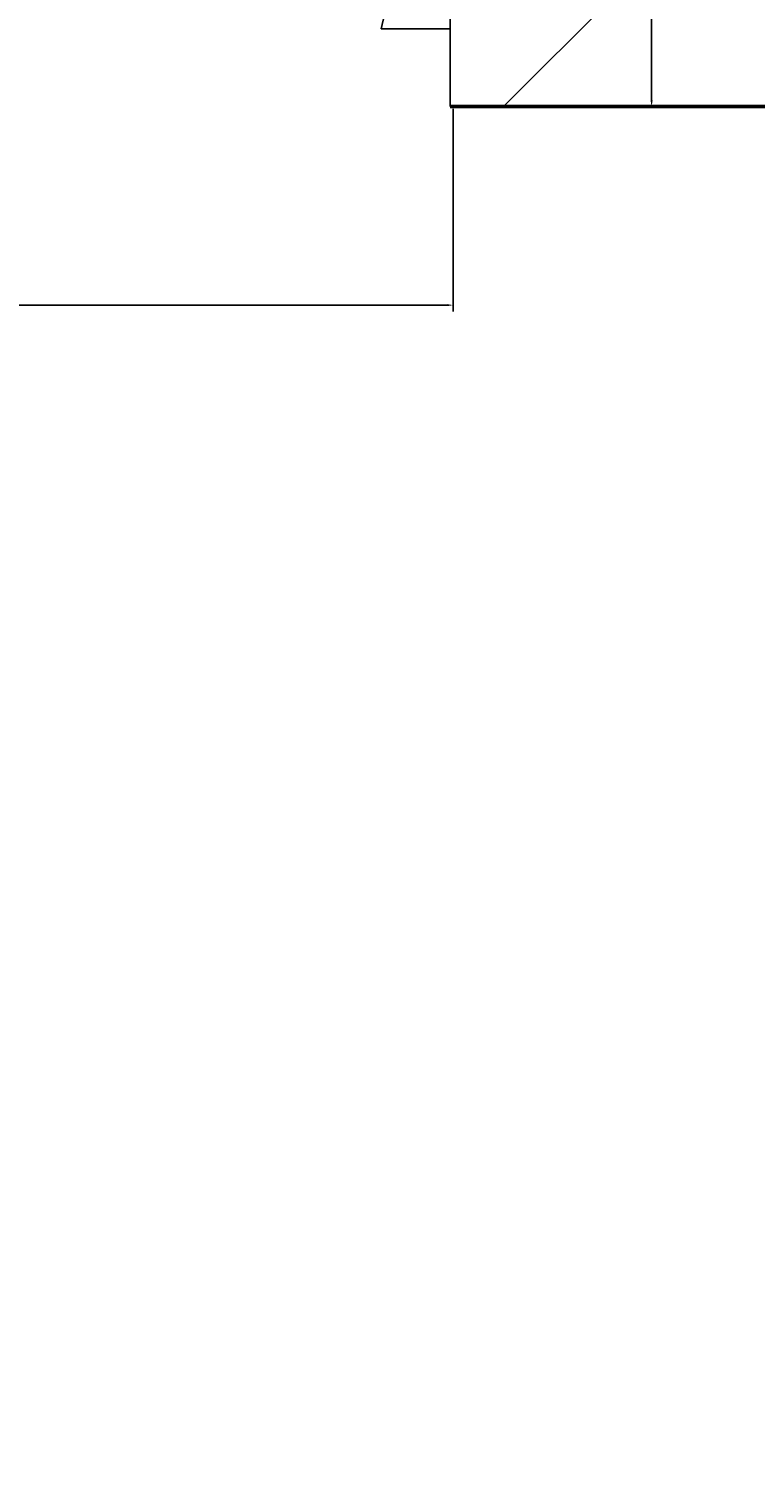
# Model space of a CAD drawing. Units: inches. Extents: x 963 to 2075, y 289 to 2657.
# Tile 93 of 98: x 1788 to 1809, y 2283 to 2325. Entities that reach past the tile are written whole.
import ezdxf

# ---------------------------------------------------------------- set-up
doc = ezdxf.new("R2010")
doc.units = ezdxf.units.IN
for name, color, linetype, lineweight in [('A-ANNO-DIMS', 2, 'Continuous', 18), ('A-DOOR', 4, 'Continuous', 25), ('A-WALL', 7, 'Continuous', 50), ('A-WALL-PATT', 8, 'Continuous', 13)]:
    doc.layers.add(name, color=color, linetype=linetype, lineweight=lineweight)
doc.styles.get("Standard").update_dxf_attribs({"font": 'arial.ttf'})
doc.dimstyles.get("Standard").update_dxf_attribs({"dimtxt": 0.18, "dimasz": 0.18, "dimexe": 0.18, "dimexo": 0.0625, "dimgap": 0.09, "dimtad": 0, "dimtih": 1, "dimtoh": 1, "dimdec": 4, "dimzin": 0, "dimdsep": 46, "dimtxsty": 'Standard', "dimcen": 0.09, "dimadec": 0, "dimazin": 0, "dimtfac": 1, "dimtdec": 4, "dimtofl": 0, "dimtmove": 0, "dimatfit": 3, "dimfxl": 1, "dimtolj": 1, "dimtzin": 0, "dimarcsym": 0})

# ---------------------------------------------------------------- blocks, each defined once
blk = doc.blocks.new('DOOR-3')
for p, q in [((2, 2.25), (2, 38.25)), ((0, 4.5), (0, 0)), ((32.386, 4.5), (32.386, 0)), ((0, 0), (0, 2.25)), ((0, 2.25), (2, 2.25)), ((32.386, 2.25), (30.386, 2.25)), ((32.386, 0), (32.386, 2.25))]:
    blk.add_line(p, q)
blk.add_arc((2, 9.059), 29.191, 346.5105, 90)
blk = doc.blocks.new('*D34')
at = {"layer": 'A-ANNO-DIMS', "color": 0, "lineweight": -2, "transparency": 16777216}
for p, q in [((1800.571, 2361.068), (1806.426, 2361.068)), ((1806.246, 2360.888), (1806.246, 2342.126)), ((1806.246, 2322.998), (1806.246, 2341.759)), ((1800.571, 2322.818), (1806.426, 2322.818))]:
    blk.add_line(p, q, dxfattribs=at)
at = {"layer": 'A-ANNO-DIMS', "color": 0, "transparency": 16777216}
for points in [[(1806.216, 2360.888), (1806.276, 2360.888), (1806.246, 2361.068)], [(1806.216, 2322.998), (1806.276, 2322.998), (1806.246, 2322.818)]]:
    blk.add_solid(points, dxfattribs=at)
at = {"layer": 'Defpoints', "color": 0, "transparency": 16777216}
for p in [(1800.508, 2361.068), (1806.246, 2361.068), (1800.508, 2322.818)]:
    blk.add_point(p, dxfattribs=at)
at = {"layer": 'A-ANNO-DIMS', "color": 0, "transparency": 16777216, "insert": (1806.246, 2341.943), "char_height": 0.18, "attachment_point": 5}
blk.add_mtext('\\A1;DOOR D3 38 TYP.', dxfattribs=at)
blk = doc.blocks.new('*D35')
at = {"layer": 'A-ANNO-DIMS', "color": 0, "lineweight": -2, "transparency": 16777216}
for p, q in [((1768.037, 2322.755), (1768.037, 2316.9)), ((1800.508, 2322.755), (1800.508, 2316.9)), ((1768.217, 2317.08), (1783.745, 2317.08)), ((1800.328, 2317.08), (1784.801, 2317.08))]:
    blk.add_line(p, q, dxfattribs=at)
at = {"layer": 'A-ANNO-DIMS', "color": 0, "transparency": 16777216}
for points in [[(1768.217, 2317.11), (1768.217, 2317.05), (1768.037, 2317.08)], [(1800.328, 2317.11), (1800.328, 2317.05), (1800.508, 2317.08)]]:
    blk.add_solid(points, dxfattribs=at)
at = {"layer": 'Defpoints', "color": 0, "transparency": 16777216}
for p in [(1768.037, 2322.818), (1800.508, 2322.818), (1800.508, 2317.08)]:
    blk.add_point(p, dxfattribs=at)
at = {"layer": 'A-ANNO-DIMS', "color": 0, "transparency": 16777216, "insert": (1784.273, 2317.08), "char_height": 0.18, "attachment_point": 5}
blk.add_mtext('\\A1;32 TYP.', dxfattribs=at)

msp = doc.modelspace()

# ---------------------------------------------------------------- hatches: boundary and pattern name
at = {"layer": 'A-WALL-PATT'}
h = msp.add_hatch(dxfattribs=at)
h.set_pattern_fill('ANSI32', color=256)
h.paths.add_polyline_path([(1296.922, 2558.318), (1203.922, 2558.318), (1203.922, 2493.818), (1191.533, 2493.818), (1191.533, 2489.318), (1211.063, 2489.318), (1211.063, 2492.02), (1211.063, 2493.818), (1208.422, 2493.818), (1208.422, 2553.818), (1292.422, 2553.818), (1292.422, 2538.863), (1296.922, 2538.863)])
h.paths.add_polyline_path([(1442.422, 2558.318), (1349.422, 2558.318), (1349.422, 2538.943), (1353.922, 2538.943), (1353.922, 2553.818), (1437.922, 2553.818), (1437.922, 2493.818), (1434.542, 2493.818), (1434.542, 2489.318), (1448.311, 2489.318), (1448.311, 2491.568), (1448.311, 2493.818), (1442.422, 2493.818)])
h.paths.add_polyline_path([(1415.554, 2491.568), (1415.554, 2493.818), (1340.941, 2493.818), (1340.941, 2489.318), (1371.922, 2489.318), (1371.922, 2378.318), (1367.596, 2378.318), (1367.596, 2373.818), (1371.922, 2373.818), (1371.922, 2355.185), (1376.422, 2355.185), (1376.422, 2489.318), (1415.554, 2489.318)])
h.paths.add_polyline_path([(1304.941, 2491.568), (1304.941, 2493.818), (1296.922, 2493.818), (1296.922, 2514.863), (1292.422, 2514.863), (1292.422, 2493.818), (1232.808, 2493.818), (1232.808, 2489.318), (1256.422, 2489.318), (1256.422, 2327.318), (1253.714, 2327.318), (1253.714, 2322.818), (1328.422, 2322.818), (1328.422, 2331.147), (1323.922, 2331.147), (1323.922, 2327.318), (1260.922, 2327.318), (1260.922, 2373.818), (1323.922, 2373.818), (1323.922, 2357.812), (1328.422, 2357.812), (1328.422, 2373.818), (1346.007, 2373.818), (1346.007, 2376.068), (1346.007, 2378.318), (1260.922, 2378.318), (1260.922, 2489.318), (1304.941, 2489.318)])
h.paths.add_polyline_path([(1226.654, 2327.318), (1124.422, 2327.318), (1124.422, 2347.447), (1119.922, 2347.447), (1119.922, 2322.818), (1163.422, 2322.818), (1163.422, 2305.435), (1165.672, 2305.435), (1167.922, 2305.435), (1167.922, 2322.818), (1226.654, 2322.818), (1226.654, 2325.068)])
h.paths.add_polyline_path([(1095.922, 2489.318), (1124.422, 2489.318), (1131.533, 2489.318), (1131.533, 2491.568), (1131.533, 2493.818), (1119.922, 2493.818), (1091.422, 2493.818), (1091.422, 2417.318), (1095.922, 2417.318), (1119.922, 2417.318), (1119.922, 2407.447), (1124.422, 2407.447), (1124.422, 2421.818), (1095.922, 2421.818)])
h.paths.add_polyline_path([(1512.922, 2558.318), (1508.422, 2558.318), (1508.422, 2493.818), (1503.401, 2493.818), (1503.401, 2489.318), (1508.422, 2489.318), (1508.422, 2327.318), (1376.422, 2327.318), (1376.422, 2330.273), (1371.922, 2330.273), (1371.922, 2298.744), (1376.422, 2298.744), (1376.422, 2322.818), (1508.422, 2322.818), (1508.422, 2165.318), (1504.255, 2165.318), (1504.255, 2160.818), (1508.422, 2160.818), (1508.422, 2108.318), (1512.922, 2108.318), (1512.922, 2160.818), (1516.182, 2160.818), (1516.182, 2163.068), (1516.182, 2165.318), (1512.922, 2165.318), (1512.922, 2322.818), (1644.922, 2322.818), (1644.922, 2298.744), (1649.422, 2298.744), (1649.422, 2322.818), (1649.422, 2330.944), (1647.172, 2330.944), (1644.922, 2330.944), (1644.922, 2327.318), (1512.922, 2327.318), (1512.922, 2489.318), (1516.759, 2489.318), (1516.759, 2491.568), (1516.759, 2493.818), (1512.922, 2493.818)])
h.paths.add_polyline_path([(1671.922, 2558.318), (1578.922, 2558.318), (1578.922, 2493.818), (1573.526, 2493.818), (1573.526, 2489.318), (1586.537, 2489.318), (1586.537, 2491.568), (1586.537, 2493.818), (1583.422, 2493.818), (1583.422, 2553.818), (1667.422, 2553.818), (1667.422, 2541.109), (1671.922, 2541.109)])
h.paths.add_polyline_path([(1681.257, 2493.818), (1671.922, 2493.818), (1671.922, 2517.109), (1667.422, 2517.109), (1667.422, 2493.818), (1610.218, 2493.818), (1610.218, 2489.318), (1644.922, 2489.318), (1644.922, 2357.865), (1649.422, 2357.865), (1649.422, 2373.818), (1652.203, 2373.818), (1652.203, 2375.827), (1652.203, 2378.318), (1649.422, 2378.318), (1649.422, 2489.318), (1681.257, 2489.318), (1681.257, 2491.568)])
h.paths.add_polyline_path([(1821.922, 2558.318), (1728.922, 2558.318), (1728.922, 2541), (1733.422, 2541), (1733.422, 2553.818), (1817.422, 2553.818), (1817.422, 2493.818), (1813.507, 2493.818), (1813.507, 2489.318), (1830.078, 2489.318), (1830.078, 2491.568), (1830.078, 2493.818), (1821.922, 2493.818)])
h.paths.add_polyline_path([(1794.244, 2493.818), (1717.257, 2493.818), (1717.257, 2489.318), (1760.422, 2489.318), (1760.422, 2378.318), (1674.401, 2378.318), (1674.401, 2373.818), (1692.922, 2373.818), (1692.922, 2356.954), (1697.422, 2356.954), (1697.422, 2373.818), (1760.422, 2373.818), (1760.422, 2327.318), (1697.422, 2327.318), (1697.422, 2333.341), (1692.922, 2333.341), (1692.922, 2322.818), (1768.037, 2322.818), (1768.037, 2325.068), (1768.037, 2327.318), (1764.922, 2327.318), (1764.922, 2489.318), (1794.244, 2489.318)])
h.paths.add_polyline_path([(1733.422, 2517), (1728.922, 2517), (1728.922, 2493.818), (1733.422, 2493.818)], flags=17)
h.paths.add_polyline_path([(1929.922, 2493.818), (1890.078, 2493.818), (1890.078, 2489.318), (1896.922, 2489.318), (1925.422, 2489.318), (1925.422, 2421.818), (1896.922, 2421.818), (1896.922, 2408.318), (1901.422, 2408.318), (1901.422, 2417.318), (1925.422, 2417.318), (1929.922, 2417.318)])
h.paths.add_polyline_path([(1901.422, 2348.318), (1896.922, 2348.318), (1896.922, 2327.318), (1800.423, 2327.318), (1800.423, 2322.818), (1853.422, 2322.818), (1853.422, 2309.453), (1857.922, 2309.453), (1857.922, 2322.818), (1901.422, 2322.818)])
h.paths.add_polyline_path([(1857.922, 2249.453), (1853.422, 2249.453), (1853.422, 2214.818), (1686.309, 2214.818), (1686.309, 2210.318), (1853.422, 2210.318), (1853.422, 2202.134), (1857.922, 2202.134), (1857.922, 2210.318)])
h.paths.add_polyline_path([(1857.922, 2142.134), (1853.422, 2142.134), (1853.422, 2115.422), (1841.422, 2115.422), (1841.422, 2088.531), (1841.422, 2046.949), (1845.922, 2046.949), (1845.922, 2110.922), (1905.922, 2110.922), (1905.922, 2092.517), (1910.422, 2092.517), (1910.422, 2115.422), (1857.922, 2115.422)])
h.paths.add_polyline_path([(1532.436, 1482.342), (1573.456, 1482.342), (1573.456, 1501), (1532.436, 1501)], flags=9)
h.paths.add_polyline_path([(1438.658, 1486.302), (1479.678, 1486.302), (1479.678, 1504.96), (1438.658, 1504.96)], flags=9)
h.paths.add_polyline_path([(1411.215, 1365.308), (1659.139, 1365.308), (1659.139, 1402.401), (1411.215, 1402.401)], flags=9)
h.paths.add_polyline_path([(1185.671, 2296.298), (1248.16, 2296.298), (1248.16, 2314.955), (1185.671, 2314.955)], flags=9)
h.paths.add_polyline_path([(1177.31, 2187.35), (1216.15, 2187.35), (1216.15, 2206.007), (1177.31, 2206.007)], flags=9)
h.paths.add_polyline_path([(1295.101, 1602.083), (1328.26, 1602.083), (1328.26, 1620.741), (1295.101, 1620.741)], flags=9)
h.paths.add_polyline_path([(1525.126, 2005.99), (1558.39, 2005.99), (1558.39, 2024.648), (1525.126, 2024.648)], flags=9)
h.paths.add_polyline_path([(1459.606, 1977.125), (1472.195, 1977.125), (1472.195, 1987.429), (1459.606, 1987.429)], flags=9)
h.paths.add_polyline_path([(1467.815, 2053.676), (1480.018, 2053.676), (1480.018, 2063.979), (1467.815, 2063.979)], flags=9)
h.paths.add_polyline_path([(1555.184, 2119.02), (1584.563, 2119.02), (1584.563, 2137.678), (1555.184, 2137.678)], flags=25)
h.paths.add_polyline_path([(1405.389, 2115.291), (1444.478, 2115.291), (1444.478, 2133.948), (1405.389, 2133.948)], flags=25)
h.paths.add_polyline_path([(1698.482, 2004.259), (1727.695, 2004.259), (1727.695, 2022.916), (1698.482, 2022.916)], flags=9)
h.paths.add_polyline_path([(1612.158, 1972.855), (1629.016, 1972.855), (1629.016, 1983.159), (1612.158, 1983.159)], flags=9)
h.paths.add_polyline_path([(1608.289, 2060.036), (1625.147, 2060.036), (1625.147, 2070.34), (1608.289, 2070.34)], flags=9)
h.paths.add_polyline_path([(1527.954, 1684.402), (1566.795, 1684.402), (1566.795, 1703.06), (1527.954, 1703.06)], flags=9)
h.paths.add_polyline_path([(1422.792, 1683.59), (1461.633, 1683.59), (1461.633, 1702.247), (1422.792, 1702.247)], flags=9)
h.paths.add_polyline_path([(1531.262, 1732.459), (1574.015, 1732.459), (1574.015, 1751.116), (1531.262, 1751.116)], flags=9)
h.paths.add_polyline_path([(1402.872, 1732.845), (1439.799, 1732.845), (1439.799, 1751.502), (1402.872, 1751.502)], flags=9)
h.paths.add_polyline_path([(1243.122, 1923.132), (1281.962, 1923.132), (1281.962, 1941.79), (1243.122, 1941.79)], flags=9)
h.paths.add_polyline_path([(1181.752, 1792.268), (1244.241, 1792.268), (1244.241, 1810.926), (1181.752, 1810.926)], flags=9)
h.paths.add_polyline_path([(1265.822, 1670.3), (1316.071, 1670.3), (1316.071, 1688.957), (1265.822, 1688.957)], flags=9)
h.paths.add_polyline_path([(1140.263, 1676.054), (1179.104, 1676.054), (1179.104, 1694.711), (1140.263, 1694.711)], flags=9)
h.paths.add_polyline_path([(1107.49, 1490.889), (1143.374, 1490.889), (1143.374, 1509.546), (1107.49, 1509.546)], flags=9)
h.paths.add_polyline_path([(1217.584, 1483.899), (1246.741, 1483.899), (1246.741, 1502.556), (1217.584, 1502.556)], flags=9)
h.paths.add_polyline_path([(1389.21, 1486.919), (1418.367, 1486.919), (1418.367, 1505.576), (1389.21, 1505.576)], flags=9)
h.paths.add_polyline_path([(1672.208, 1602.083), (1705.366, 1602.083), (1705.366, 1620.741), (1672.208, 1620.741)], flags=9)
h.paths.add_polyline_path([(1752.082, 1522.638), (1781.24, 1522.638), (1781.24, 1541.295), (1752.082, 1541.295)], flags=9)
h.paths.add_polyline_path([(1848.275, 1491.26), (1884.158, 1491.26), (1884.158, 1509.918), (1848.275, 1509.918)], flags=9)
h.paths.add_polyline_path([(1822.47, 1685.62), (1861.31, 1685.62), (1861.31, 1704.278), (1822.47, 1704.278)], flags=9)
h.paths.add_polyline_path([(1713.195, 1672.232), (1763.444, 1672.232), (1763.444, 1690.889), (1713.195, 1690.889)], flags=9)
h.paths.add_polyline_path([(1736.619, 1790.578), (1799.109, 1790.578), (1799.109, 1809.235), (1736.619, 1809.235)], flags=9)
h.paths.add_polyline_path([(1691.491, 1916.355), (1730.332, 1916.355), (1730.332, 1935.013), (1691.491, 1935.013)], flags=9)
h.paths.add_polyline_path([(1764.872, 1973.922), (1794.306, 1973.922), (1794.306, 1992.58), (1764.872, 1992.58)], flags=9)
h.paths.add_polyline_path([(1767.854, 2034.017), (1797.288, 2034.017), (1797.288, 2052.674), (1767.854, 2052.674)], flags=9)
h.paths.add_polyline_path([(1851.593, 2060.331), (1880.751, 2060.331), (1880.751, 2078.989), (1851.593, 2078.989)], flags=25)
h.paths.add_polyline_path([(1688.491, 2086.874), (1727.332, 2086.874), (1727.332, 2105.531), (1688.491, 2105.531)], flags=9)
h.paths.add_polyline_path([(1537.743, 2293.581), (1580.495, 2293.581), (1580.495, 2312.239), (1537.743, 2312.239)], flags=25)
h.paths.add_polyline_path([(1425.587, 2296.109), (1468.34, 2296.109), (1468.34, 2314.766), (1425.587, 2314.766)], flags=25)
h.paths.add_polyline_path([(1278.518, 2004.184), (1307.72, 2004.184), (1307.72, 2022.841), (1278.518, 2022.841)], flags=9)
h.paths.add_polyline_path([(1193.282, 1973.635), (1222.715, 1973.635), (1222.715, 1992.292), (1193.282, 1992.292)], flags=9)
h.paths.add_polyline_path([(1192.411, 2040.577), (1221.845, 2040.577), (1221.845, 2059.234), (1192.411, 2059.234)], flags=9)
h.paths.add_polyline_path([(1130.603, 1951.393), (1159.76, 1951.393), (1159.76, 1970.05), (1130.603, 1970.05)], flags=9)
h.paths.add_polyline_path([(1132.827, 2052.494), (1161.984, 2052.494), (1161.984, 2071.151), (1132.827, 2071.151)], flags=9)
h.paths.add_polyline_path([(1265.128, 2334.619), (1315.377, 2334.619), (1315.377, 2353.277), (1265.128, 2353.277)], flags=25)
h.paths.add_polyline_path([(1136.741, 2330.785), (1175.582, 2330.785), (1175.582, 2349.443), (1136.741, 2349.443)], flags=9)
h.paths.add_polyline_path([(1287.422, 2417.204), (1320.58, 2417.204), (1320.58, 2435.861), (1287.422, 2435.861)], flags=25)
h.paths.add_polyline_path([(1430.988, 2329.159), (1469.828, 2329.159), (1469.828, 2347.816), (1430.988, 2347.816)], flags=25)
h.paths.add_polyline_path([(1525.424, 2329.213), (1564.264, 2329.213), (1564.264, 2347.87), (1525.424, 2347.87)], flags=25)
h.paths.add_polyline_path([(1684.525, 2382.799), (1717.683, 2382.799), (1717.683, 2401.457), (1684.525, 2401.457)], flags=25)
h.paths.add_polyline_path([(1704.805, 2340.293), (1755.054, 2340.293), (1755.054, 2358.95), (1704.805, 2358.95)], flags=25)
h.paths.add_polyline_path([(1694.113, 2287.757), (1756.602, 2287.757), (1756.602, 2306.414), (1694.113, 2306.414)], flags=9)
h.paths.add_polyline_path([(1815.778, 2329.861), (1854.618, 2329.861), (1854.618, 2348.518), (1815.778, 2348.518)], flags=9)
h.paths.add_polyline_path([(1842.873, 2514.256), (1878.756, 2514.256), (1878.756, 2532.914), (1842.873, 2532.914)], flags=9)
h.paths.add_polyline_path([(1769.513, 2531.447), (1798.671, 2531.447), (1798.671, 2550.104), (1769.513, 2550.104)], flags=25)
h.paths.add_polyline_path([(1594.772, 2518.468), (1623.93, 2518.468), (1623.93, 2537.125), (1594.772, 2537.125)], flags=25)
h.paths.add_polyline_path([(1520.723, 2516.185), (1556.606, 2516.185), (1556.606, 2534.842), (1520.723, 2534.842)], flags=25)
h.paths.add_polyline_path([(1464.456, 2516.694), (1500.34, 2516.694), (1500.34, 2535.351), (1464.456, 2535.351)], flags=25)
h.paths.add_polyline_path([(1365.696, 2528.97), (1394.854, 2528.97), (1394.854, 2547.627), (1365.696, 2547.627)], flags=25)
h.paths.add_polyline_path([(1222.838, 2516.231), (1251.995, 2516.231), (1251.995, 2534.889), (1222.838, 2534.889)], flags=25)
h.paths.add_polyline_path([(1104.545, 2509.6), (1140.429, 2509.6), (1140.429, 2528.257), (1104.545, 2528.257)], flags=9)

# ---------------------------------------------------------------- linework, layer by layer
at = {"layer": 'A-WALL'}
msp.add_line((1800.423, 2322.818), (1853.422, 2322.818), dxfattribs=at)

# ---------------------------------------------------------------- block references
at = {"layer": 'A-DOOR'}
msp.add_blockref('DOOR-3', (1768.037, 2322.818), dxfattribs=at)

# ---------------------------------------------------------------- dimensions: what is measured, and where the dimension line sits
at = {"layer": 'A-ANNO-DIMS'}
dim = msp.add_linear_dim(base=(1806.246, 2361.068), p1=(1800.508, 2322.818), p2=(1800.508, 2361.068), angle=90, text='DOOR D3 <> TYP.', dimstyle='Standard', override={"dimdec": 0, "dimlfac": 1, "dimrnd": 0, "dimzin": 0, "dimdsep": 46, "dimlunit": 2}, dxfattribs=at)
dim.commit()
dim.dimension.update_dxf_attribs({"geometry": '*D34', "text_midpoint": (1806.246, 2341.943)})
dim = msp.add_linear_dim(base=(1800.508, 2317.08), p1=(1768.037, 2322.818), p2=(1800.508, 2322.818), text='<> TYP.', dimstyle='Standard', override={"dimdec": 0, "dimlfac": 1, "dimrnd": 0, "dimzin": 0, "dimdsep": 46, "dimlunit": 2}, dxfattribs=at)
dim.commit()
dim.dimension.update_dxf_attribs({"geometry": '*D35', "text_midpoint": (1784.273, 2317.08)})

doc.saveas('drawing.dxf')
